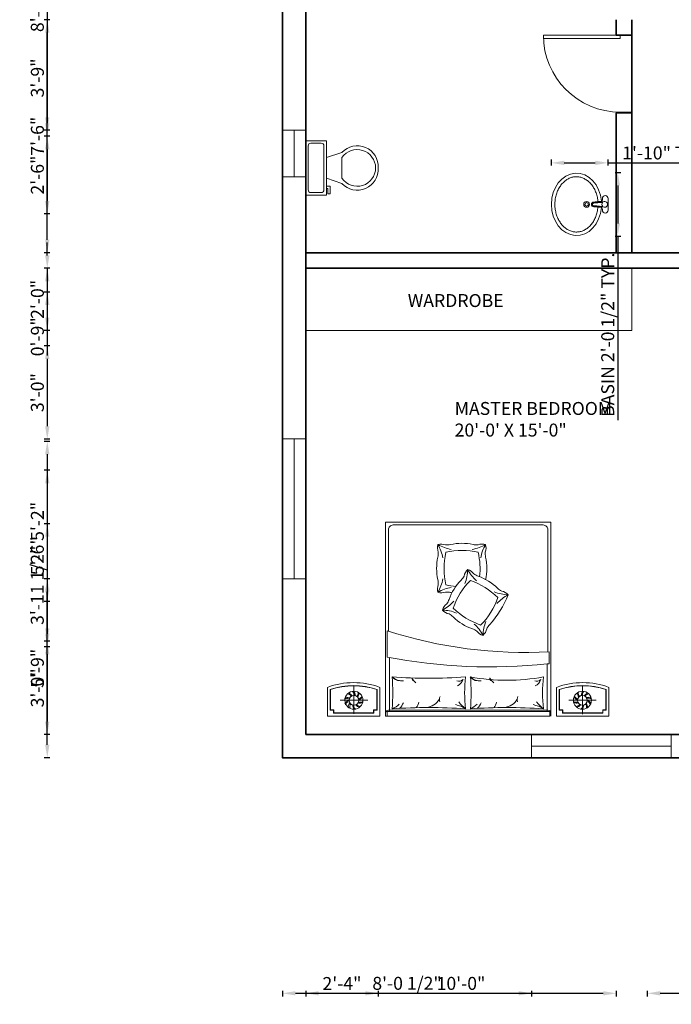
# Model space of a CAD drawing. Units: inches. Extents: x -100 to 766, y -562 to 63.
# Tile 1 of 11: x -100 to 152, y -562 to -182. Entities that reach past the tile are written whole.
import ezdxf

# ---------------------------------------------------------------- set-up
doc = ezdxf.new("R2010")
doc.units = ezdxf.units.IN
for name, color, linetype, lineweight in [('A-ANNO-DIMS', 2, 'Continuous', 18), ('A-ANNO-TEXT', 7, 'Continuous', 18), ('A-AREA-IDEN', 7, 'Continuous', 18), ('A-DOOR', 3, 'Continuous', 18), ('A-FLOR-CASE', 32, 'Continuous', 18), ('A-FLOR-FIXT', 8, 'Continuous', 18), ('A-GLAZ', 4, 'Continuous', 18), ('A-WALL', 7, 'Continuous', 35), ('furn', 8, 'Continuous', 13)]:
    doc.layers.add(name, color=color, linetype=linetype, lineweight=lineweight)
doc.styles.get("Standard").update_dxf_attribs({"font": 'arial.ttf'})
doc.dimstyles.new('ISO-25', dxfattribs={"dimtxt": 5, "dimasz": 5, "dimexe": 1.25, "dimexo": 0.625, "dimtad": 1, "dimlunit": 3, "dimtxsty": 'Standard', "dimcen": 2.5, "dimadec": 0, "dimazin": 0, "dimtfac": 1, "dimtmove": 0, "dimatfit": 3, "dimfxl": 1, "dimfxlon": 1, "dimarcsym": 0})

# ---------------------------------------------------------------- blocks, each defined once
blk = doc.blocks.new('*U2')
for p, q in [((0, 0), (0, -6)), ((40, 0), (40, -6))]:
    blk.add_line(p, q)
blk.add_lwpolyline([(0, 0), (0, 40), (1.75, 40), (1.75, 0)], close=True)
blk.add_arc((0, 0), 40, 0, 90)
blk = doc.blocks.new('*U4')
for p, q in [((9.5, -6), (9.5, -2)), ((-10, -8.5), (-8, -8.5)), ((-10, -9.5), (-10, -8.5)), ((-7, -9.5), (-10, -9.5)), ((-8, -8.5), (-8, -8)), ((-7, -8), (-7, -9.5)), ((-4, -8), (-6, -14)), ((4, -8), (6, -14)), ((4, -14), (-4, -14))]:
    blk.add_line(p, q)
blk.add_lwpolyline([(10.5, -8), (10.5, 0), (-10.5, 0), (-10.5, -8)], close=True)
for points in [[(-9.5, -2), (-9.5, -6)], [(8.5, -1), (-8.5, -1)], [(-8.5, -7), (8.5, -7)]]:
    blk.add_lwpolyline(points)
for centre, radius, start, end in [((-8.625, -1.875), 0.8839, 81.8699, 188.1301), ((8.625, -1.875), 0.8839, 351.8699, 98.1301), ((-8.625, -6.125), 0.8839, 171.869898, 278.1301), ((8.625, -6.125), 0.8839, 261.8699, 8.1301), ((-0.4772, -19.9188), 8.0953, 133.01722, 273.38), ((0.0374, -19.8731), 7.127, 124.50543, 269.7), ((-0.0373, -19.8731), 7.127, 270.3, 55.4946), ((0.4773, -19.9188), 8.0953, 266.62, 46.9828)]:
    blk.add_arc(centre, radius, start, end)
blk = doc.blocks.new('A$C359865C9')
for p, q in [((0.26, 0.586), (0.38, 0.586)), ((0.26, 0.526), (0.272, 0.526)), ((0.368, 0.526), (0.381, 0.526))]:
    blk.add_line(p, q)
for radius in [0.03, 0.018]:
    blk.add_circle((0.32, 0.363), radius)
for centre, radius, start, end in [((0.26, 0.556), 0.03, 90.0061, 270.0061), ((0.272, 0.508), 0.018, 0.0061, 90.0061), ((0.32, 0.55), 0.03, 348.1537, 191.8463), ((0.32, 0.55), 0.03, 222.4523, 317.5477), ((0.368, 0.508), 0.018, 90.0061, 180.0061), ((0.38, 0.556), 0.03, 270.0061, 89.9816), ((0.32, 0.436), 0.024, 180.0061, 0.0061), ((0.32, 0.436), 0.0204, 180.0061, 0.0061), ((0.32, 0.436), 0.0144, 180.0061, 0.0061)]:
    blk.add_arc(centre, radius, start, end)
at = {"ltscale": 100, "extrusion": (0, 0, -1)}
blk.add_ellipse((0.32, 0.258), major_axis=(0.322, 0), ratio=0.80597, start_param=-1.471508, end_param=4.612925, dxfattribs=at)
at = {"extrusion": (0, 0, -1)}
blk.add_ellipse((0.32, 0.583), major_axis=(-0.00812, 0), ratio=0.392595, dxfattribs=at)
for points, knots in [([(0.291, 0.543), (0.295, 0.498), (0.295, 0.491), (0.296, 0.476), (0.297, 0.469), (0.298, 0.454), (0.299, 0.446), (0.3, 0.438), (0.3, 0.437), (0.3, 0.436)], [2.511178, 2.511178, 2.511178, 2.511178, 20.495008, 20.495008, 39.297594, 39.297594, 58.10018, 58.10018, 60.208758, 60.208758, 60.208758, 60.208758]), ([(0.298, 0.529), (0.298, 0.528), (0.298, 0.527), (0.299, 0.518), (0.299, 0.513), (0.301, 0.499), (0.301, 0.493), (0.301, 0.488), (0.302, 0.487), (0.302, 0.486), (0.302, 0.485), (0.302, 0.483), (0.302, 0.481), (0.303, 0.476), (0.303, 0.472), (0.304, 0.462), (0.304, 0.457), (0.305, 0.446), (0.305, 0.441), (0.306, 0.437)], [4.643985, 4.643985, 4.643985, 4.643985, 5.282102, 5.282102, 8.976667, 8.976667, 16.365798, 16.365798, 18.536065, 18.536065, 20.434607, 20.434607, 24.231692, 24.231692, 34.371999, 34.371999, 47.807513, 47.807513, 60.208758, 60.208758, 60.208758, 60.208758]), ([(0.342, 0.529), (0.342, 0.528), (0.342, 0.527), (0.341, 0.518), (0.341, 0.513), (0.34, 0.499), (0.339, 0.493), (0.339, 0.488), (0.339, 0.487), (0.338, 0.486), (0.338, 0.485), (0.338, 0.483), (0.338, 0.481), (0.338, 0.476), (0.337, 0.472), (0.336, 0.462), (0.336, 0.457), (0.335, 0.446), (0.335, 0.441), (0.334, 0.437)], [4.643985, 4.643985, 4.643985, 4.643985, 5.282102, 5.282102, 8.976667, 8.976667, 16.365798, 16.365798, 18.536065, 18.536065, 20.434607, 20.434607, 24.231692, 24.231692, 34.371999, 34.371999, 47.807513, 47.807513, 60.208758, 60.208758, 60.208758, 60.208758]), ([(0.349, 0.543), (0.346, 0.498), (0.345, 0.491), (0.344, 0.476), (0.343, 0.469), (0.342, 0.454), (0.341, 0.446), (0.341, 0.438), (0.341, 0.437), (0.34, 0.436)], [2.511178, 2.511178, 2.511178, 2.511178, 20.495008, 20.495008, 39.297594, 39.297594, 58.10018, 58.10018, 60.208758, 60.208758, 60.208758, 60.208758]), ([(0.348, 0.48), (0.348, 0.48), (0.348, 0.48), (0.365, 0.479), (0.381, 0.476), (0.414, 0.469), (0.429, 0.465), (0.459, 0.453), (0.474, 0.446), (0.501, 0.431), (0.513, 0.423), (0.536, 0.404), (0.547, 0.394), (0.565, 0.373), (0.573, 0.362), (0.586, 0.339), (0.592, 0.328), (0.6, 0.304), (0.603, 0.291), (0.606, 0.267), (0.606, 0.255), (0.604, 0.23), (0.601, 0.218), (0.594, 0.194), (0.589, 0.182), (0.577, 0.16), (0.569, 0.149), (0.552, 0.127), (0.542, 0.117), (0.52, 0.099), (0.508, 0.09), (0.482, 0.074), (0.469, 0.067), (0.44, 0.055), (0.424, 0.05), (0.393, 0.042), (0.377, 0.039), (0.344, 0.035), (0.327, 0.034), (0.294, 0.035), (0.278, 0.037), (0.245, 0.042), (0.229, 0.046), (0.199, 0.056), (0.184, 0.061), (0.156, 0.075), (0.143, 0.083), (0.118, 0.1), (0.107, 0.109), (0.087, 0.129), (0.078, 0.139), (0.062, 0.161), (0.056, 0.172), (0.045, 0.196), (0.041, 0.208), (0.036, 0.232), (0.035, 0.244), (0.034, 0.257), (0.034, 0.257), (0.034, 0.258), (0.034, 0.266), (0.035, 0.275), (0.038, 0.296), (0.041, 0.308), (0.05, 0.332), (0.056, 0.343), (0.07, 0.366), (0.078, 0.377), (0.097, 0.398), (0.108, 0.408), (0.131, 0.426), (0.144, 0.434), (0.171, 0.449), (0.186, 0.455), (0.216, 0.466), (0.232, 0.471), (0.263, 0.477), (0.278, 0.479), (0.293, 0.48)], [1.664851, 1.664851, 1.664851, 1.664851, 1.666804, 1.666804, 1.838807, 1.838807, 2.01081, 2.01081, 2.182814, 2.182814, 2.354817, 2.354817, 2.52682, 2.52682, 2.698824, 2.698824, 2.870827, 2.870827, 3.04283, 3.04283, 3.214834, 3.214834, 3.384783, 3.384783, 3.554732, 3.554732, 3.724681, 3.724681, 3.89463, 3.89463, 4.064578, 4.064578, 4.234527, 4.234527, 4.404476, 4.404476, 4.574425, 4.574425, 4.744374, 4.744374, 4.914323, 4.914323, 5.084272, 5.084272, 5.254221, 5.254221, 5.42417, 5.42417, 5.594119, 5.594119, 5.764068, 5.764068, 5.934016, 5.934016, 6.103965, 6.103965, 6.273914, 6.273914, 6.283185, 6.283185, 6.283185, 6.401959, 6.401959, 6.573962, 6.573962, 6.745965, 6.745965, 6.917969, 6.917969, 7.089972, 7.089972, 7.261975, 7.261975, 7.433979, 7.433979, 7.605982, 7.605982, 7.759676, 7.759676, 7.759676, 7.759676]), ([(0.29, 0.508), (0.291, 0.494), (0.294, 0.47), (0.295, 0.446), (0.296, 0.436)], [0, 0, 0, 0, 35.358253, 60.208758, 60.208758, 60.208758, 60.208758]), ([(0.35, 0.508), (0.349, 0.494), (0.347, 0.47), (0.345, 0.446), (0.344, 0.436)], [0, 0, 0, 0, 35.358253, 60.208758, 60.208758, 60.208758, 60.208758])]:
    blk.add_open_spline(points, degree=3, knots=knots)
blk = doc.blocks.new('WIN-54IN')
blk.add_line((4.5, 54), (4.5, 0))
blk.add_lwpolyline([(0, 54), (9, 54), (9, 0), (0, 0)], close=True)
blk = doc.blocks.new('WIN-18IN')
blk.add_line((4.5, 18), (4.5, 0))
blk.add_lwpolyline([(0, 18), (9, 18), (9, 0), (0, 0)], close=True)
blk = doc.blocks.new('BED-DOUBLE-WITH-NIGHTSTANDS')
for p, q in [((23.96, 1.73), (23.96, 22.55)), ((84.9, 1.73), (84.9, 20.16)), ((10.25, 11.43), (10.25, 0.8)), ((98.58, 11.43), (98.58, 0.79)), ((4.93, 6.11), (15.57, 6.11)), ((103.9, 6.11), (93.26, 6.11)), ((85.22, 2.28), (23.61, 2.28))]:
    blk.add_line(p, q)
for points in [[(86.32, 0), (86.32, 74.89), (22.5, 74.89), (22.5, 0)], [(2.43, 1.11), (2.43, 2.44), (1.11, 2.44)], [(2.32, 1.11), (2.32, 2.32), (1.11, 2.32)], [(2.32, 1.22), (17.97, 1.22)], [(2.32, 1.11), (17.97, 1.11)], [(17.85, 1.11), (17.85, 2.44), (19.18, 2.44)], [(17.97, 1.11), (17.97, 2.32), (19.18, 2.32)], [(23.1, 0), (23.1, 1.73), (85.95, 1.73), (85.95, 0), (22.5, 0)], [(90.97, 1.11), (90.97, 2.44), (89.64, 2.44)], [(90.86, 1.11), (90.86, 2.33), (89.64, 2.33)], [(106.5, 1.22), (90.86, 1.22)], [(106.5, 1.11), (90.86, 1.11)], [(106.39, 1.11), (106.39, 2.44), (107.72, 2.44)], [(106.5, 1.11), (106.5, 2.33), (107.72, 2.33)]]:
    blk.add_lwpolyline(points)
for points in [[(85.22, 24.82), (85.22, 71.94, 0.414214), (83.37, 73.78), (25.45, 73.78, 0.414214), (23.61, 71.94), (23.61, 32.78)], [(42.71, 66.24, 0.159461), (42.84, 63.34, -0.076283), (42.71, 61.4, 0.115075), (42.71, 52.64, -0.076283), (42.84, 50.7, 0.159461), (42.71, 47.8)], [(44.62, 61.06, 0.091296), (42.71, 66.24, 0.091296), (47.89, 64.35)], [(55.97, 64.35, 0.091296), (61.15, 66.24, 0.091296), (59.25, 61.06, 0.091296)], [(58.24, 63.23, 0.111006), (45.84, 63.22, 0.119549), (45.84, 50.66, 0.033212), (49.65, 50.08)], [(54.24, 56.57, 0.159461), (52.81, 54.04, -0.076283), (51.68, 52.46, 0.115075), (47.05, 45.03, -0.076283), (46.13, 43.32, 0.159461), (44.49, 40.92)], [(53.12, 51.17, 0.091296), (54.24, 56.57, 0.091296), (57.64, 52.23)], [(47.89, 49.69, 0.091296), (42.71, 47.8, 0.091296), (44.62, 52.98, 0.091296)], [(65.83, 45.8, 0.111006), (55.29, 52.35, 0.119549), (48.65, 41.69, 0.107813), (59.16, 35.11)], [(59.21, 35.12, 0.121865), (65.83, 45.8, 0.121865)], [(64.49, 47.96, 0.091296), (69.89, 46.82, 0.091296), (65.54, 43.43, 0.091296)], [(49.89, 39.78, 0.091296), (44.49, 40.92, 0.091296), (48.84, 44.31, 0.091296)], [(61.26, 36.57, 0.091296), (60.14, 31.16, 0.091296), (56.74, 35.51, 0.091296)], [(19.18, 2.32), (19.18, 10.3, 0.167087), (1.11, 10.3), (1.11, 2.32)], [(19.07, 2.32), (19.07, 10.22, 0.165559), (1.22, 10.22), (1.22, 2.32)], [(89.64, 2.33), (89.64, 10.3, -0.167087), (107.72, 10.3), (107.72, 2.33)], [(89.75, 2.33), (89.75, 10.22, -0.165559), (107.61, 10.22), (107.61, 2.33)]]:
    blk.add_lwpolyline(points, format="xyb")
for points in [[(85.77, 20.16), (84.9, 20.16, -0.072944), (23.1, 22.73), (23.1, 32.96, 0.092568), (85.77, 24.85)], [(0, 11.07), (0, 0), (20.29, 0), (20.29, 11.07, 0.181818)], [(53.41, 15.12, 0.058596), (53.41, 2.79, 0.036648), (24.98, 2.79, 0.052163), (24.98, 15.12, 0.036967)], [(83.49, 15.12, 0.058596), (83.49, 2.79, 0.036889), (55.25, 2.79, 0.052163), (55.25, 15.12, 0.093111)], [(108.83, 11.07), (108.83, 0), (88.54, 0), (88.54, 11.07, -0.181818)]]:
    blk.add_lwpolyline(points, format="xyb", close=True)
for centre, radius in [((10.25, 6.11), 3.48), ((10.25, 6.11), 1.88), ((98.58, 6.11), 3.48), ((98.58, 6.11), 1.88)]:
    blk.add_circle(centre, radius)
for centre, radius, start, end in [((43.85, 61.01), 5.35, 70.7023, 102.284), ((46.15, 72.45), 6.4, 265.2252, 282.6741), ((51.99, 47.44), 19.27, 77.0576, 103.3153), ((57.67, 72.48), 6.4, 257.6988, 275.1477), ((59.91, 61.73), 4.68, 74.5791, 110.8198), ((56.65, 64.98), 4.68, 339.3666, 15.6073), ((32.87, 56.89), 26.15, 353.1956, 14.0284), ((67.41, 62.78), 6.4, 175.0387, 192.4877), ((42.38, 57.02), 19.27, 346.8711, 13.1289), ((52.44, 51.53), 5.35, 38.7754, 70.3571), ((60.44, 60.02), 6.4, 233.2983, 250.7472), ((52.18, 35.71), 19.27, 45.1307, 71.3884), ((44.09, 51.89), 4.32, 251.3996, 291.5774), ((46.25, 41.5), 6.4, 77.6988, 95.1477), ((51.93, 66.54), 19.27, 257.0576, 258.7033), ((32.5, 62.1), 40.4, 318.3818, 337.7644), ((70.24, 53.96), 6.4, 225.7718, 243.2208), ((66.46, 43.65), 4.68, 42.6522, 78.8929), ((47.82, 43.66), 4.32, 219.4726, 259.6505), ((44.16, 33.7), 6.4, 45.7718, 63.2208), ((62.22, 51.95), 19.27, 225.1307, 251.3884), ((67.28, 30.79), 6.4, 135.5854, 153.0343), ((53.96, 27.63), 6.4, 53.2983, 70.7472), ((61.38, 35.5), 4.51, 217.2937, 254.0973), ((56.98, 34.61), 4.68, 312.4658, 348.7065), ((27.82, 16.88), 3.19, 213.6349, 270.8456), ((28.76, 18.64), 5.04, 224.406, 276.8342), ((33.7, 14.59), 1.03, 173.7543, 257.2187), ((45.1, 23.69), 15.4, 216.2085, 225.0849), ((50.68, 16.26), 2.8, 256.4823, 308.5563), ((48.55, 15.4), 4.1, 294.2916, 340.9896), ((58.85, 18.64), 5.04, 224.406, 276.8342), ((57.9, 16.88), 3.19, 213.6349, 270.8456), ((63.79, 14.59), 1.03, 173.7543, 257.2187), ((75.18, 23.69), 15.4, 216.2085, 225.0849), ((80.77, 16.26), 2.8, 256.4823, 308.5563), ((78.64, 15.4), 4.1, 294.2916, 340.9896), ((7.79, 6.82), 1.7, 31.462, 91.6998), ((7.68, 6.63), 2.23, 33.5103, 79.83), ((8.68, 8.13), 1.7, 355.462, 55.6998), ((8.47, 8.04), 2.23, 357.5103, 43.83), ((10.16, 8.67), 1.7, 319.462, 19.6998), ((9.94, 8.72), 2.23, 321.5103, 7.83), ((11.68, 8.23), 1.7, 283.462, 343.6998), ((97.15, 8.23), 1.7, 196.3002, 256.538), ((98.88, 8.72), 2.23, 172.17, 218.4897), ((98.67, 8.67), 1.7, 160.3002, 220.538), ((100.36, 8.04), 2.23, 136.17, 182.4897), ((100.15, 8.13), 1.7, 124.3002, 184.538), ((101.15, 6.63), 2.23, 100.17, 146.4897), ((101.03, 6.82), 1.7, 88.3002, 148.538), ((7.59, 5.14), 1.7, 67.462, 127.6998), ((7.62, 4.92), 2.23, 69.5103, 115.83), ((8.72, 3.73), 2.23, 105.5103, 151.83), ((8.57, 3.9), 1.7, 103.462, 163.6998), ((10.3, 3.42), 2.23, 141.5103, 187.83), ((10.34, 3.56), 1.7, 139.462, 199.6998), ((12.03, 4.19), 2.23, 177.5103, 223.83), ((11.82, 4.1), 1.7, 175.462, 235.6998), ((12.82, 5.6), 2.23, 213.5103, 259.83), ((12.71, 5.41), 1.7, 211.462, 271.6998), ((12.63, 7.21), 2.23, 249.5103, 295.83), ((12.65, 6.99), 1.7, 247.462, 307.6998), ((11.53, 8.4), 2.23, 285.5103, 331.83), ((21.28, 11.24), 9.3, 294.6457, 314.1585), ((24.5, 6.89), 5.16, 310.5354, 340.3558), ((30.57, 6.21), 4.8, 321.8174, 349.8987), ((37.48, 10.1), 6.84, 276.6849, 328.3182), ((46.36, 6.29), 3.06, 155.8927, 196.1192), ((46.85, -7.52), 12.22, 57.5379, 77.5233), ((62.65, 14.32), 14.78, 216.4935, 231.2792), ((51.37, 11.24), 9.3, 294.6457, 314.1585), ((54.59, 6.89), 5.16, 310.5354, 340.3558), ((60.65, 6.21), 4.8, 321.8174, 349.8987), ((67.57, 10.1), 6.84, 276.6849, 328.3182), ((76.44, 6.29), 3.06, 155.8927, 196.1192), ((76.94, -7.52), 12.22, 57.5379, 77.5233), ((92.74, 14.32), 14.78, 216.4935, 231.2792), ((96.17, 6.99), 1.7, 232.3002, 292.538), ((96.2, 7.21), 2.23, 244.17, 290.4897), ((97.3, 8.4), 2.23, 208.17, 254.4897), ((96.12, 5.41), 1.7, 268.3002, 328.538), ((96.01, 5.6), 2.23, 280.17, 326.4897), ((97, 4.1), 1.7, 304.3002, 4.538), ((96.8, 4.19), 2.23, 316.17, 2.4897), ((98.49, 3.56), 1.7, 340.3002, 40.538), ((98.27, 3.51), 2.23, 352.17, 38.4897), ((100.96, 5.02), 2.23, 64.17, 110.4897), ((100.98, 5.24), 1.7, 52.3002, 112.538), ((100, 3.99), 1.7, 16.3002, 76.538), ((99.86, 3.83), 2.23, 28.17, 74.4897), ((23.61, 1.17), 1.11, 90, 180), ((85.22, 1.17), 1.11, 0, 90)]:
    blk.add_arc(centre, radius, start, end)
blk = doc.blocks.new('*D28')
at = {"layer": 'A-ANNO-DIMS', "color": 0, "lineweight": -2, "transparency": 16777216}
for p, q in [((129.95, -241.2), (132.2, -241.2)), ((130.95, -246.2), (130.95, -260.85)), ((129.95, -265.85), (132.2, -265.85)), ((130.95, -265.85), (130.95, -336.91))]:
    blk.add_line(p, q, dxfattribs=at)
at = {"layer": 'A-ANNO-DIMS', "color": 0, "transparency": 16777216}
for points in [[(130.12, -246.2), (131.79, -246.2), (130.95, -241.2)], [(130.12, -260.85), (131.79, -260.85), (130.95, -265.85)]]:
    blk.add_solid(points, dxfattribs=at)
at = {"layer": 'Defpoints', "color": 0, "transparency": 16777216}
for p in [(127.26, -241.2), (127.26, -265.85), (130.95, -265.85)]:
    blk.add_point(p, dxfattribs=at)
at = {"layer": 'A-ANNO-DIMS', "color": 0, "transparency": 16777216, "insert": (127.74, -303.88), "char_height": 5, "attachment_point": 5, "rotation": 90}
blk.add_mtext('BASIN 2\'-0 1/2" TYP.', dxfattribs=at)
blk = doc.blocks.new('*D29')
at = {"layer": 'A-ANNO-DIMS', "color": 0, "lineweight": -2, "transparency": 16777216}
for p, q in [((105.31, -238.5), (105.31, -236.25)), ((110.31, -237.5), (122.26, -237.5)), ((127.26, -238.5), (127.26, -236.25)), ((127.26, -237.5), (167.4, -237.5))]:
    blk.add_line(p, q, dxfattribs=at)
at = {"layer": 'A-ANNO-DIMS', "color": 0, "transparency": 16777216}
for points in [[(110.31, -236.67), (110.31, -238.34), (105.31, -237.5)], [(122.26, -236.67), (122.26, -238.34), (127.26, -237.5)]]:
    blk.add_solid(points, dxfattribs=at)
at = {"layer": 'Defpoints', "color": 0, "transparency": 16777216}
for p in [(127.26, -237.5), (105.31, -241.2), (127.26, -241.2)]:
    blk.add_point(p, dxfattribs=at)
at = {"layer": 'A-ANNO-DIMS', "color": 0, "transparency": 16777216, "insert": (149.83, -234.33), "char_height": 5, "attachment_point": 5}
blk.add_mtext('1\'-10" TYP.', dxfattribs=at)
blk = doc.blocks.new('*D40')
at = {"layer": 'A-ANNO-DIMS', "color": 0, "lineweight": -2, "transparency": 16777216}
for p, q in [((142.39, -557.16), (142.39, -559.41)), ((147.39, -558.16), (209.39, -558.16)), ((214.39, -557.16), (214.39, -559.41))]:
    blk.add_line(p, q, dxfattribs=at)
at = {"layer": 'A-ANNO-DIMS', "color": 0, "transparency": 16777216}
for points in [[(147.39, -557.32), (147.39, -558.99), (142.39, -558.16)], [(209.39, -557.32), (209.39, -558.99), (214.39, -558.16)]]:
    blk.add_solid(points, dxfattribs=at)
at = {"layer": 'Defpoints', "color": 0, "transparency": 16777216}
for p in [(142.39, -56.21), (214.39, -56.21), (214.39, -558.16)]:
    blk.add_point(p, dxfattribs=at)
at = {"layer": 'A-ANNO-DIMS', "color": 0, "transparency": 16777216, "insert": (178.39, -554.98), "char_height": 5, "attachment_point": 5}
blk.add_mtext('6\'-0"', dxfattribs=at)
blk = doc.blocks.new('*D42')
at = {"layer": 'A-ANNO-DIMS', "color": 0, "lineweight": -2, "transparency": 16777216}
for p, q in [((10.39, -557.16), (10.39, -559.41)), ((15.39, -558.16), (125.39, -558.16)), ((130.39, -557.16), (130.39, -559.41))]:
    blk.add_line(p, q, dxfattribs=at)
at = {"layer": 'A-ANNO-DIMS', "color": 0, "transparency": 16777216}
for points in [[(15.39, -557.32), (15.39, -558.99), (10.39, -558.16)], [(125.39, -557.32), (125.39, -558.99), (130.39, -558.16)]]:
    blk.add_solid(points, dxfattribs=at)
at = {"layer": 'Defpoints', "color": 0, "transparency": 16777216}
for p in [(10.39, -182.21), (130.39, -182.21), (130.39, -558.16)]:
    blk.add_point(p, dxfattribs=at)
at = {"layer": 'A-ANNO-DIMS', "color": 0, "transparency": 16777216, "insert": (70.39, -554.98), "char_height": 5, "attachment_point": 5}
blk.add_mtext('10\'-0"', dxfattribs=at)
blk = doc.blocks.new('*D43')
at = {"layer": 'A-ANNO-DIMS', "color": 0, "lineweight": -2, "transparency": 16777216}
for p, q in [((-88.51, -182.21), (-90.76, -182.21)), ((-89.51, -267.21), (-89.51, -187.21)), ((-88.51, -272.21), (-90.76, -272.21))]:
    blk.add_line(p, q, dxfattribs=at)
at = {"layer": 'A-ANNO-DIMS', "color": 0, "transparency": 16777216}
for points in [[(-90.35, -187.21), (-88.68, -187.21), (-89.51, -182.21)], [(-90.35, -267.21), (-88.68, -267.21), (-89.51, -272.21)]]:
    blk.add_solid(points, dxfattribs=at)
at = {"layer": 'Defpoints', "color": 0, "transparency": 16777216}
for p in [(-89.51, -182.21), (10.39, -182.21), (10.39, -272.21)]:
    blk.add_point(p, dxfattribs=at)
at = {"layer": 'A-ANNO-DIMS', "color": 0, "transparency": 16777216, "insert": (-92.69, -227.21), "char_height": 5, "attachment_point": 5, "rotation": 90}
blk.add_mtext('7\'-6"', dxfattribs=at)
blk = doc.blocks.new('*D48')
at = {"layer": 'A-ANNO-DIMS', "color": 0, "lineweight": -2, "transparency": 16777216}
for p, q in [((-88.51, -227.21), (-90.76, -227.21)), ((-89.51, -232.21), (-89.51, -252.21)), ((-88.51, -257.21), (-90.76, -257.21))]:
    blk.add_line(p, q, dxfattribs=at)
at = {"layer": 'A-ANNO-DIMS', "color": 0, "transparency": 16777216}
for points in [[(-90.35, -232.21), (-88.68, -232.21), (-89.51, -227.21)], [(-90.35, -252.21), (-88.68, -252.21), (-89.51, -257.21)]]:
    blk.add_solid(points, dxfattribs=at)
at = {"layer": 'Defpoints', "color": 0, "transparency": 16777216}
for p in [(562.39, -227.21), (-89.51, -257.21), (562.39, -257.21)]:
    blk.add_point(p, dxfattribs=at)
at = {"layer": 'A-ANNO-DIMS', "color": 0, "transparency": 16777216, "insert": (-92.69, -242.21), "char_height": 5, "attachment_point": 5, "rotation": 90}
blk.add_mtext('2\'-6"', dxfattribs=at)
blk = doc.blocks.new('*D49')
at = {"layer": 'A-ANNO-DIMS', "color": 0, "lineweight": -2, "transparency": 16777216}
for p, q in [((-88.51, -356.21), (-90.76, -356.21)), ((-89.51, -361.21), (-89.51, -417.21)), ((-88.51, -422.21), (-90.76, -422.21))]:
    blk.add_line(p, q, dxfattribs=at)
at = {"layer": 'A-ANNO-DIMS', "color": 0, "transparency": 16777216}
for points in [[(-90.35, -361.21), (-88.68, -361.21), (-89.51, -356.21)], [(-90.35, -417.21), (-88.68, -417.21), (-89.51, -422.21)]]:
    blk.add_solid(points, dxfattribs=at)
at = {"layer": 'Defpoints', "color": 0, "transparency": 16777216}
for p in [(562.39, -356.21), (-89.51, -422.21), (562.39, -422.21)]:
    blk.add_point(p, dxfattribs=at)
at = {"layer": 'A-ANNO-DIMS', "color": 0, "transparency": 16777216, "insert": (-92.69, -389.21), "char_height": 5, "attachment_point": 5, "rotation": 90}
blk.add_mtext('5\'-6"', dxfattribs=at)
blk = doc.blocks.new('*D51')
at = {"layer": 'A-ANNO-DIMS', "color": 0, "lineweight": -2, "transparency": 16777216}
for p, q in [((-88.51, -308.21), (-90.76, -308.21)), ((-89.51, -313.21), (-89.51, -339.21)), ((-88.51, -344.21), (-90.76, -344.21))]:
    blk.add_line(p, q, dxfattribs=at)
at = {"layer": 'A-ANNO-DIMS', "color": 0, "transparency": 16777216}
for points in [[(-90.35, -313.21), (-88.68, -313.21), (-89.51, -308.21)], [(-90.35, -339.21), (-88.68, -339.21), (-89.51, -344.21)]]:
    blk.add_solid(points, dxfattribs=at)
at = {"layer": 'Defpoints', "color": 0, "transparency": 16777216}
for p in [(598.6, -308.21), (-89.51, -344.21), (598.6, -344.21)]:
    blk.add_point(p, dxfattribs=at)
at = {"layer": 'A-ANNO-DIMS', "color": 0, "transparency": 16777216, "insert": (-92.69, -326.21), "char_height": 5, "attachment_point": 5, "rotation": 90}
blk.add_mtext('3\'-0"', dxfattribs=at)
blk = doc.blocks.new('*D53')
at = {"layer": 'A-ANNO-DIMS', "color": 0, "lineweight": -2, "transparency": 16777216}
for p, q in [((-88.51, -278.21), (-90.76, -278.21)), ((-89.51, -283.21), (-89.51, -297.21)), ((-88.51, -302.21), (-90.76, -302.21))]:
    blk.add_line(p, q, dxfattribs=at)
at = {"layer": 'A-ANNO-DIMS', "color": 0, "transparency": 16777216}
for points in [[(-90.35, -283.21), (-88.68, -283.21), (-89.51, -278.21)], [(-90.35, -297.21), (-88.68, -297.21), (-89.51, -302.21)]]:
    blk.add_solid(points, dxfattribs=at)
at = {"layer": 'Defpoints', "color": 0, "transparency": 16777216}
for p in [(10.39, -278.21), (-89.51, -302.21), (10.39, -302.21)]:
    blk.add_point(p, dxfattribs=at)
at = {"layer": 'A-ANNO-DIMS', "color": 0, "transparency": 16777216, "insert": (-92.69, -290.21), "char_height": 5, "attachment_point": 5, "rotation": 90}
blk.add_mtext('2\'-0"', dxfattribs=at)
blk = doc.blocks.new('*D60')
at = {"layer": 'A-ANNO-DIMS', "color": 0, "lineweight": -2, "transparency": 16777216}
for p, q in [((-88.51, -118.48), (-90.76, -118.48)), ((-89.51, -123.48), (-89.51, -219.89)), ((-88.51, -224.89), (-90.76, -224.89))]:
    blk.add_line(p, q, dxfattribs=at)
at = {"layer": 'A-ANNO-DIMS', "color": 0, "transparency": 16777216}
for points in [[(-90.35, -123.48), (-88.68, -123.48), (-89.51, -118.48)], [(-90.35, -219.89), (-88.68, -219.89), (-89.51, -224.89)]]:
    blk.add_solid(points, dxfattribs=at)
at = {"layer": 'Defpoints', "color": 0, "transparency": 16777216}
for p in [(1.39, -118.48), (-89.51, -224.89), (1.39, -224.89)]:
    blk.add_point(p, dxfattribs=at)
at = {"layer": 'A-ANNO-DIMS', "color": 0, "transparency": 16777216, "insert": (-92.72, -171.69), "char_height": 5, "attachment_point": 5, "rotation": 90}
blk.add_mtext('8\'-10 1/2"', dxfattribs=at)
blk = doc.blocks.new('*D61')
at = {"layer": 'A-ANNO-DIMS', "color": 0, "lineweight": -2, "transparency": 16777216}
for p, q in [((-88.51, -398.12), (-90.76, -398.12)), ((-89.51, -462.21), (-89.51, -403.12)), ((-88.51, -467.21), (-90.76, -467.21))]:
    blk.add_line(p, q, dxfattribs=at)
at = {"layer": 'A-ANNO-DIMS', "color": 0, "transparency": 16777216}
for points in [[(-90.35, -403.12), (-88.68, -403.12), (-89.51, -398.12)], [(-90.35, -462.21), (-88.68, -462.21), (-89.51, -467.21)]]:
    blk.add_solid(points, dxfattribs=at)
at = {"layer": 'Defpoints', "color": 0, "transparency": 16777216}
for p in [(-89.51, -398.12), (1.39, -398.12), (1.39, -467.21)]:
    blk.add_point(p, dxfattribs=at)
at = {"layer": 'A-ANNO-DIMS', "color": 0, "transparency": 16777216, "insert": (-92.69, -432.66), "char_height": 5, "attachment_point": 5, "rotation": 90}
blk.add_mtext('5\'-9"', dxfattribs=at)
blk = doc.blocks.new('*D65')
at = {"layer": 'A-ANNO-DIMS', "color": 0, "lineweight": -2, "transparency": 16777216}
for p, q in [((1.39, -557.16), (1.39, -559.41)), ((6.39, -558.16), (92.67, -558.16)), ((97.67, -557.16), (97.67, -559.41))]:
    blk.add_line(p, q, dxfattribs=at)
at = {"layer": 'A-ANNO-DIMS', "color": 0, "transparency": 16777216}
for points in [[(6.39, -557.32), (6.39, -558.99), (1.39, -558.16)], [(92.67, -557.32), (92.67, -558.99), (97.67, -558.16)]]:
    blk.add_solid(points, dxfattribs=at)
at = {"layer": 'Defpoints', "color": 0, "transparency": 16777216}
for p in [(1.39, -467.21), (97.67, -467.19), (97.67, -558.16)]:
    blk.add_point(p, dxfattribs=at)
at = {"layer": 'A-ANNO-DIMS', "color": 0, "transparency": 16777216, "insert": (49.53, -554.95), "char_height": 5, "attachment_point": 5}
blk.add_mtext('8\'-0 1/2"', dxfattribs=at)
blk = doc.blocks.new('*D70')
at = {"layer": 'A-ANNO-DIMS', "color": 0, "lineweight": -2, "transparency": 16777216}
for p, q in [((-88.51, -376.85), (-90.76, -376.85)), ((-89.51, -381.85), (-89.51, -419.34)), ((-88.51, -424.34), (-90.76, -424.34))]:
    blk.add_line(p, q, dxfattribs=at)
at = {"layer": 'A-ANNO-DIMS', "color": 0, "transparency": 16777216}
for points in [[(-90.35, -381.85), (-88.68, -381.85), (-89.51, -376.85)], [(-90.35, -419.34), (-88.68, -419.34), (-89.51, -424.34)]]:
    blk.add_solid(points, dxfattribs=at)
at = {"layer": 'Defpoints', "color": 0, "transparency": 16777216}
for p in [(679.5, -376.85), (-89.51, -424.34), (679.5, -424.34)]:
    blk.add_point(p, dxfattribs=at)
at = {"layer": 'A-ANNO-DIMS', "color": 0, "transparency": 16777216, "insert": (-92.73, -400.59), "char_height": 5, "attachment_point": 5, "rotation": 90}
blk.add_mtext('3\'-11 1/2"', dxfattribs=at)
blk = doc.blocks.new('*D73')
at = {"layer": 'A-ANNO-DIMS', "color": 0, "lineweight": -2, "transparency": 16777216}
for p, q in [((-88.51, -345.04), (-90.76, -345.04)), ((-89.51, -350.04), (-89.51, -401.82)), ((-88.51, -406.82), (-90.76, -406.82))]:
    blk.add_line(p, q, dxfattribs=at)
at = {"layer": 'A-ANNO-DIMS', "color": 0, "transparency": 16777216}
for points in [[(-90.35, -350.04), (-88.68, -350.04), (-89.51, -345.04)], [(-90.35, -401.82), (-88.68, -401.82), (-89.51, -406.82)]]:
    blk.add_solid(points, dxfattribs=at)
at = {"layer": 'Defpoints', "color": 0, "transparency": 16777216}
for p in [(475.3, -345.04), (-89.51, -406.82), (475.3, -406.82)]:
    blk.add_point(p, dxfattribs=at)
at = {"layer": 'A-ANNO-DIMS', "color": 0, "transparency": 16777216, "insert": (-92.69, -375.93), "char_height": 5, "attachment_point": 5, "rotation": 90}
blk.add_mtext('5\'-2"', dxfattribs=at)
blk = doc.blocks.new('*D76')
at = {"layer": 'A-ANNO-DIMS', "color": 0, "lineweight": -2, "transparency": 16777216}
for p, q in [((760.28, -228.95), (762.53, -228.95)), ((761.28, -233.95), (761.28, -244.95)), ((760.28, -249.95), (762.53, -249.95))]:
    blk.add_line(p, q, dxfattribs=at)
at = {"layer": 'A-ANNO-DIMS', "color": 0, "transparency": 16777216}
for points in [[(760.45, -233.95), (762.11, -233.95), (761.28, -228.95)], [(760.45, -244.95), (762.11, -244.95), (761.28, -249.95)]]:
    blk.add_solid(points, dxfattribs=at)
at = {"layer": 'Defpoints', "color": 0, "transparency": 16777216}
for p in [(10.38, -228.95), (10.38, -249.95), (761.28, -249.95)]:
    blk.add_point(p, dxfattribs=at)
at = {"layer": 'A-ANNO-DIMS', "color": 0, "transparency": 16777216, "insert": (758.1, -239.45), "char_height": 5, "attachment_point": 5, "rotation": 90}
blk.add_mtext('1\'-9"', dxfattribs=at)
blk = doc.blocks.new('*D77')
at = {"layer": 'A-ANNO-DIMS', "color": 0, "lineweight": -2, "transparency": 16777216}
for p, q in [((10.38, -557.16), (10.38, -559.41)), ((15.38, -558.16), (33.38, -558.16)), ((38.38, -557.16), (38.38, -559.41))]:
    blk.add_line(p, q, dxfattribs=at)
at = {"layer": 'A-ANNO-DIMS', "color": 0, "transparency": 16777216}
for points in [[(15.38, -557.32), (15.38, -558.99), (10.38, -558.16)], [(33.38, -557.32), (33.38, -558.99), (38.38, -558.16)]]:
    blk.add_solid(points, dxfattribs=at)
at = {"layer": 'Defpoints', "color": 0, "transparency": 16777216}
for p in [(38.38, -239.45), (10.38, -249.95), (38.38, -558.16)]:
    blk.add_point(p, dxfattribs=at)
at = {"layer": 'A-ANNO-DIMS', "color": 0, "transparency": 16777216, "insert": (24.38, -555.02), "char_height": 5, "attachment_point": 5}
blk.add_mtext('2\'-4"', dxfattribs=at)
blk = doc.blocks.new('*D81')
at = {"layer": 'A-ANNO-DIMS', "color": 0, "lineweight": -2, "transparency": 16777216}
for p, q in [((-89.51, -273.21), (-89.51, -268.21)), ((-88.51, -278.21), (-90.76, -278.21)), ((-89.51, -278.21), (-89.51, -287.38)), ((-88.51, -287.38), (-90.76, -287.38)), ((-89.51, -292.38), (-89.51, -311.92))]:
    blk.add_line(p, q, dxfattribs=at)
at = {"layer": 'A-ANNO-DIMS', "color": 0, "transparency": 16777216}
for points in [[(-90.35, -273.21), (-88.68, -273.21), (-89.51, -278.21)], [(-90.35, -292.38), (-88.68, -292.38), (-89.51, -287.38)]]:
    blk.add_solid(points, dxfattribs=at)
at = {"layer": 'Defpoints', "color": 0, "transparency": 16777216}
for p in [(412.39, -278.21), (-89.51, -287.38), (412.39, -287.38)]:
    blk.add_point(p, dxfattribs=at)
at = {"layer": 'A-ANNO-DIMS', "color": 0, "transparency": 16777216, "insert": (-92.69, -304.65), "char_height": 5, "attachment_point": 5, "rotation": 90}
blk.add_mtext('0\'-9"', dxfattribs=at)
blk = doc.blocks.new('*D82')
at = {"layer": 'A-ANNO-DIMS', "color": 0, "lineweight": -2, "transparency": 16777216}
for p, q in [((-88.51, -182.21), (-90.76, -182.21)), ((-89.51, -187.21), (-89.51, -222.21)), ((-88.51, -227.21), (-90.76, -227.21))]:
    blk.add_line(p, q, dxfattribs=at)
at = {"layer": 'A-ANNO-DIMS', "color": 0, "transparency": 16777216}
for points in [[(-90.35, -187.21), (-88.68, -187.21), (-89.51, -182.21)], [(-90.35, -222.21), (-88.68, -222.21), (-89.51, -227.21)]]:
    blk.add_solid(points, dxfattribs=at)
at = {"layer": 'Defpoints', "color": 0, "transparency": 16777216}
for p in [(562.39, -182.21), (-89.51, -227.21), (562.39, -227.21)]:
    blk.add_point(p, dxfattribs=at)
at = {"layer": 'A-ANNO-DIMS', "color": 0, "transparency": 16777216, "insert": (-92.69, -204.71), "char_height": 5, "attachment_point": 5, "rotation": 90}
blk.add_mtext('3\'-9"', dxfattribs=at)
blk = doc.blocks.new('*D83')
at = {"layer": 'A-ANNO-DIMS', "color": 0, "lineweight": -2, "transparency": 16777216}
for p, q in [((-88.51, -422.21), (-90.76, -422.21)), ((-89.51, -427.21), (-89.51, -453.21)), ((-88.51, -458.21), (-90.76, -458.21))]:
    blk.add_line(p, q, dxfattribs=at)
at = {"layer": 'A-ANNO-DIMS', "color": 0, "transparency": 16777216}
for points in [[(-90.35, -427.21), (-88.68, -427.21), (-89.51, -422.21)], [(-90.35, -453.21), (-88.68, -453.21), (-89.51, -458.21)]]:
    blk.add_solid(points, dxfattribs=at)
at = {"layer": 'Defpoints', "color": 0, "transparency": 16777216}
for p in [(562.39, -422.21), (-89.51, -458.21), (562.39, -458.21)]:
    blk.add_point(p, dxfattribs=at)
at = {"layer": 'A-ANNO-DIMS', "color": 0, "transparency": 16777216, "insert": (-92.69, -440.21), "char_height": 5, "attachment_point": 5, "rotation": 90}
blk.add_mtext('3\'-0"', dxfattribs=at)
blk = doc.blocks.new('*D85')
at = {"layer": 'A-ANNO-DIMS', "color": 0, "lineweight": -2, "transparency": 16777216}
for p, q in [((761.28, -177.21), (761.28, -172.21)), ((760.28, -182.21), (762.53, -182.21)), ((761.28, -182.21), (761.28, -188.21)), ((760.28, -188.21), (762.53, -188.21)), ((761.28, -193.21), (761.28, -212.76))]:
    blk.add_line(p, q, dxfattribs=at)
at = {"layer": 'A-ANNO-DIMS', "color": 0, "transparency": 16777216}
for points in [[(760.45, -177.21), (762.11, -177.21), (761.28, -182.21)], [(760.45, -193.21), (762.11, -193.21), (761.28, -188.21)]]:
    blk.add_solid(points, dxfattribs=at)
at = {"layer": 'Defpoints', "color": 0, "transparency": 16777216}
for p in [(130.39, -182.21), (130.39, -188.21), (761.28, -188.21)]:
    blk.add_point(p, dxfattribs=at)
at = {"layer": 'A-ANNO-DIMS', "color": 0, "transparency": 16777216, "insert": (758.1, -205.49), "char_height": 5, "attachment_point": 5, "rotation": 90}
blk.add_mtext('0\'-6"', dxfattribs=at)

msp = doc.modelspace()

# ---------------------------------------------------------------- linework, layer by layer
at = {"layer": 'A-FLOR-CASE'}
for p in [(136.388, -278.214), (10.388, -302.214)]:
    msp.add_line(p, (136.388, -302.214), dxfattribs=at)
at = {"layer": 'A-WALL'}
for p, q in [((10.388, -458.214), (10.388, 3.786)), ((130.388, -188.214), (130.388, -182.214)), ((136.388, -272.214), (136.388, -182.214)), ((136.388, -188.214), (130.388, -188.214)), ((130.388, -272.214), (130.388, -218.214)), ((136.388, -218.214), (130.388, -218.214)), ((250.388, -272.214), (10.388, -272.214)), ((172.344, -278.214), (10.388, -278.214)), ((250.388, -458.214), (10.388, -458.214))]:
    msp.add_line(p, q, dxfattribs=at)
msp.add_lwpolyline([(1.388, 12.786), (721.388, 12.786), (721.388, -467.214), (1.388, -467.214)], close=True, dxfattribs=at)

# ---------------------------------------------------------------- block references
at = {"layer": 'A-DOOR', "xscale": -0.7422758465611929, "yscale": 0.7422758465611929, "zscale": 0.7422758465611929, "rotation": 90}
msp.add_blockref('*U2', (131.934, -188.214), dxfattribs=at)
at = {"layer": 'A-FLOR-FIXT', "rotation": 89.99999999999999}
msp.add_blockref('*U4', (10.379, -239.449), dxfattribs=at)
at = {"layer": 'A-FLOR-FIXT', "xscale": 37.38131337077302, "yscale": 37.38131337077302, "zscale": 37.38131337077302, "rotation": 270}
msp.add_blockref('A$C359865C9', (105.359, -241.563), dxfattribs=at)
at = {"layer": 'A-GLAZ'}
for name, p in [('WIN-18IN', (1.388, -242.892)), ('WIN-54IN', (1.388, -398.115))]:
    msp.add_blockref(name, p, dxfattribs=at)
at = {"layer": 'A-GLAZ', "rotation": 270}
msp.add_blockref('WIN-54IN', (97.67, -458.194), dxfattribs=at)
at = {"layer": 'furn'}
msp.add_blockref('BED-DOUBLE-WITH-NIGHTSTANDS', (18.745, -451.1), dxfattribs=at)

# ---------------------------------------------------------------- texts
at = {"layer": 'A-ANNO-TEXT', "insert": (49.809, -288.166), "char_height": 5, "attachment_point": 1}
msp.add_mtext_dynamic_manual_height_columns('WARDROBE', width=41.4154, gutter_width=12.5, heights=[0], dxfattribs=at)
at = {"layer": 'A-AREA-IDEN', "insert": (67.919, -329.833), "char_height": 5, "attachment_point": 1}
msp.add_mtext_dynamic_manual_height_columns('MASTER BEDROOM\\P20\'-0\' X 15\'-0"', width=80.98818, gutter_width=12.5, heights=[0], dxfattribs=at)

# ---------------------------------------------------------------- dimensions: what is measured, and where the dimension line sits
at = {"layer": 'A-ANNO-DIMS'}
for base, p1, p2, picture, middle in [((214.388, -558.156), (142.388, -56.214), (214.388, -56.214), '*D40', (178.388, -554.979)), ((130.388, -558.156), (10.388, -182.214), (130.388, -182.214), '*D42', (70.388, -554.979)), ((38.379, -558.156), (10.379, -249.949), (38.379, -239.449), '*D77', (24.379, -555.021)), ((97.67, -558.156), (1.388, -467.214), (97.67, -467.193), '*D65', (49.529, -554.946))]:
    dim = msp.add_linear_dim(base=base, p1=p1, p2=p2, dimstyle='ISO-25', override={"dimdec": 1, "dimlfac": 1, "dimrnd": 0, "dimzin": 1, "dimdsep": 46, "dimlunit": 4, "dimfrac": 2}, dxfattribs=at)
    dim.commit()
    dim.dimension.update_dxf_attribs({"geometry": picture, "text_midpoint": middle})
for base, p1, p2, picture, middle in [((-89.513, -224.892), (1.388, -118.484), (1.388, -224.892), '*D60', (-92.723, -171.688)), ((761.28, -188.214), (130.388, -182.214), (130.388, -188.214), '*D85', (758.102, -205.485)), ((-89.513, -227.214), (562.394, -182.214), (562.394, -227.214), '*D82', (-92.693, -204.714)), ((-89.513, -182.214), (10.388, -272.214), (10.388, -182.214), '*D43', (-92.691, -227.214)), ((-89.513, -257.214), (562.394, -227.214), (562.394, -257.214), '*D48', (-92.691, -242.214)), ((761.28, -249.949), (10.379, -228.949), (10.379, -249.949), '*D76', (758.102, -239.449)), ((-89.513, -287.377), (412.394, -278.214), (412.394, -287.377), '*D81', (-92.691, -304.648)), ((-89.513, -302.214), (10.388, -278.214), (10.388, -302.214), '*D53', (-92.691, -290.214)), ((-89.513, -344.214), (598.603, -308.214), (598.603, -344.214), '*D51', (-92.693, -326.214)), ((-89.513, -406.822), (475.3, -345.045), (475.3, -406.822), '*D73', (-92.691, -375.933)), ((-89.513, -422.214), (562.394, -356.214), (562.394, -422.214), '*D49', (-92.691, -389.214)), ((-89.513, -424.336), (679.495, -376.848), (679.495, -424.336), '*D70', (-92.725, -400.592)), ((-89.513, -398.115), (1.388, -467.214), (1.388, -398.115), '*D61', (-92.691, -432.665)), ((-89.513, -458.214), (562.394, -422.214), (562.394, -458.214), '*D83', (-92.693, -440.214))]:
    dim = msp.add_linear_dim(base=base, p1=p1, p2=p2, angle=90, dimstyle='ISO-25', override={"dimdec": 1, "dimlfac": 1, "dimrnd": 0, "dimzin": 1, "dimdsep": 46, "dimlunit": 4, "dimfrac": 2}, dxfattribs=at)
    dim.commit()
    dim.dimension.update_dxf_attribs({"geometry": picture, "text_midpoint": middle})
dim = msp.add_linear_dim(base=(127.257, -237.504), p1=(105.312, -241.202), p2=(127.257, -241.202), text='<> TYP.', dimstyle='ISO-25', override={"dimdec": 1, "dimlfac": 1, "dimrnd": 0, "dimzin": 1, "dimdsep": 46, "dimlunit": 4, "dimfrac": 2}, dxfattribs=at)
dim.commit()
dim.dimension.update_dxf_attribs({"geometry": '*D29', "text_midpoint": (149.828, -234.327)})
dim = msp.add_linear_dim(base=(130.955, -265.853), p1=(127.257, -241.202), p2=(127.257, -265.853), angle=270, text='BASIN <> TYP.', dimstyle='ISO-25', override={"dimdec": 1, "dimlfac": 1, "dimrnd": 0, "dimzin": 1, "dimdsep": 46, "dimlunit": 4, "dimfrac": 2}, dxfattribs=at)
dim.commit()
dim.dimension.update_dxf_attribs({"geometry": '*D28', "text_midpoint": (127.745, -303.882)})

doc.saveas('drawing.dxf')
